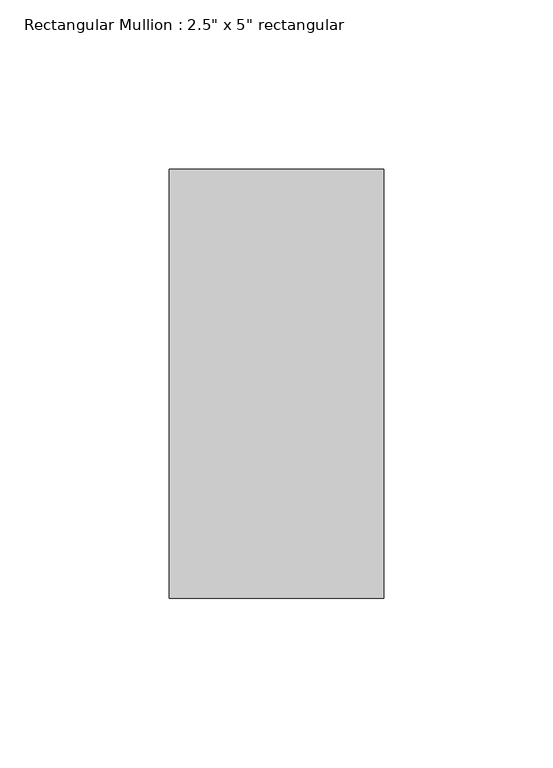
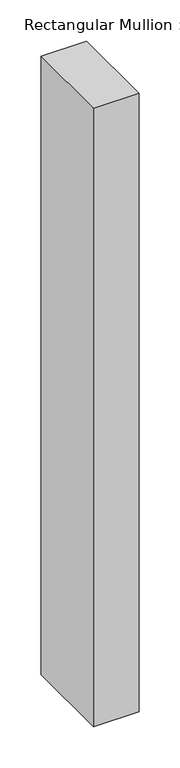
"""IFC4 building model written with IfcOpenShell, lengths in millimetres: member geometry."""

from ifc_helpers import new_model, si_unit, frame, origin, place, context, project, spatial, polyline, outline, extrude, source, transform, mapped, element, save


def member_73c23c35(model_context):
    return source(origin(), model_context, "Body", "SweptSolid", [
        extrude(outline(polyline([(0.0, 63.5), (0.0, -63.5), (-63.5, -63.5), (-63.5, 63.5), (0.0, 63.5)])), frame((0.0, 0.0, -914.4), z_axis=(0.0, 0.0, 1.0), x_axis=(1.0, 0.0, 0.0)), (0.0, 0.0, 1.0), 914.4),
    ])


if __name__ == "__main__":
    model = new_model("IFC4")
    model_context = context("Model", 3, world=origin())
    ifc_project = project(units=[si_unit("LENGTHUNIT", "METRE", prefix="MILLI")], contexts=[model_context])
    site = spatial("IfcSite", under=ifc_project)
    building = spatial("IfcBuilding", under=site)
    placement = place(None, origin())
    member_shape = member_73c23c35(model_context)
    element("IfcMember", 1, ObjectType="Rectangular Mullion : 2.5\" x 5\" rectangular", at=placement, inside=building, context=model_context, shape_type="MappedRepresentation", body=[
        mapped(member_shape, transform((0.0, 0.0, 0.0), x_axis=(1.0, 0.0, 0.0), y_axis=(0.0, 1.0, 0.0), z_axis=(0.0, 0.0, 1.0))),
    ])
    save(model, "model.ifc")

# Revit data of these elements
# Type "Rectangular Mullion : 2.5\" x 5\" rectangular"
#   built-in parameter 1007304 = 0.416667 (stored number, unit not read)
#   built-in parameter 1007301 = 0.104167 (stored number, unit not read)
#   built-in parameter 1007300 = 0.104167 (stored number, unit not read)
# Element 1 (IfcMember, "Rectangular Mullion : 2.5\" x 5\" rectangular")
#   Materials on its faces: "metal black"
# Materials
#   "metal black": class "Generic", colour RGB 120 120 120, transparency 0, Cost = 0
